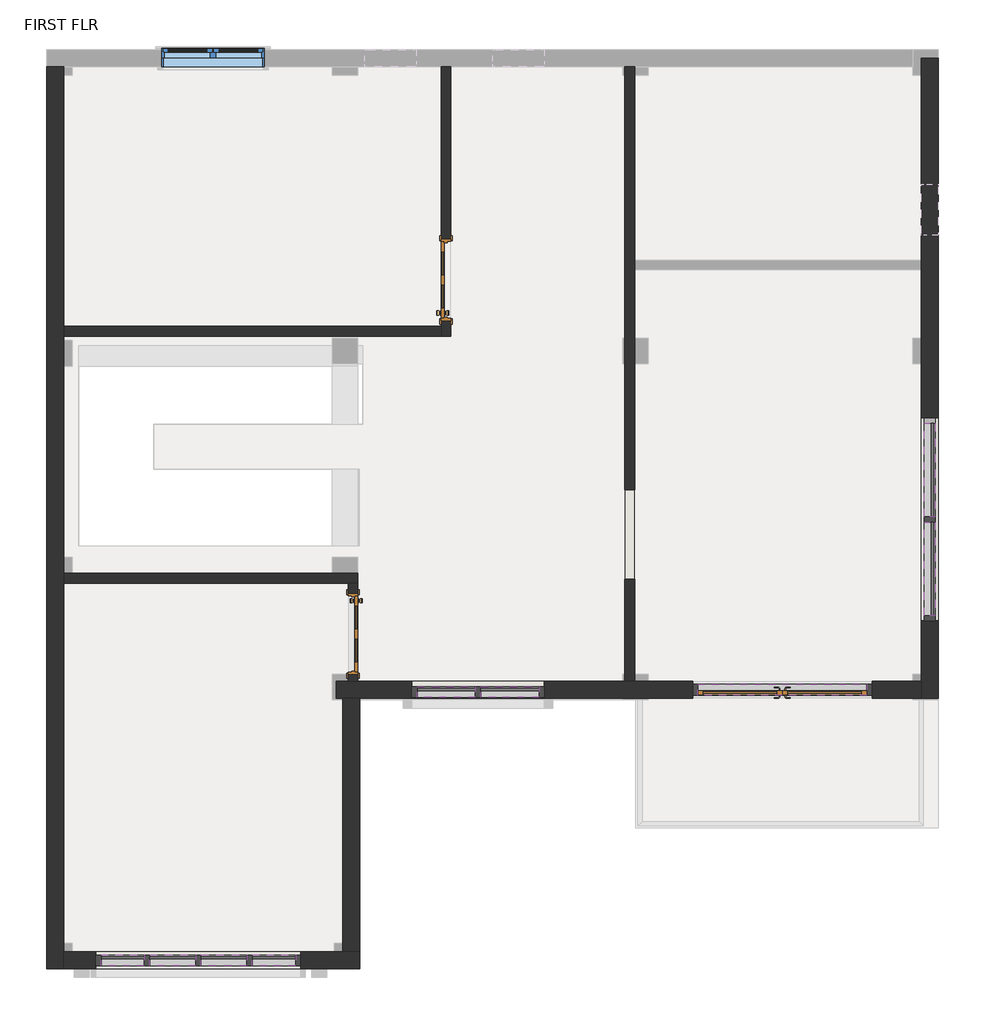
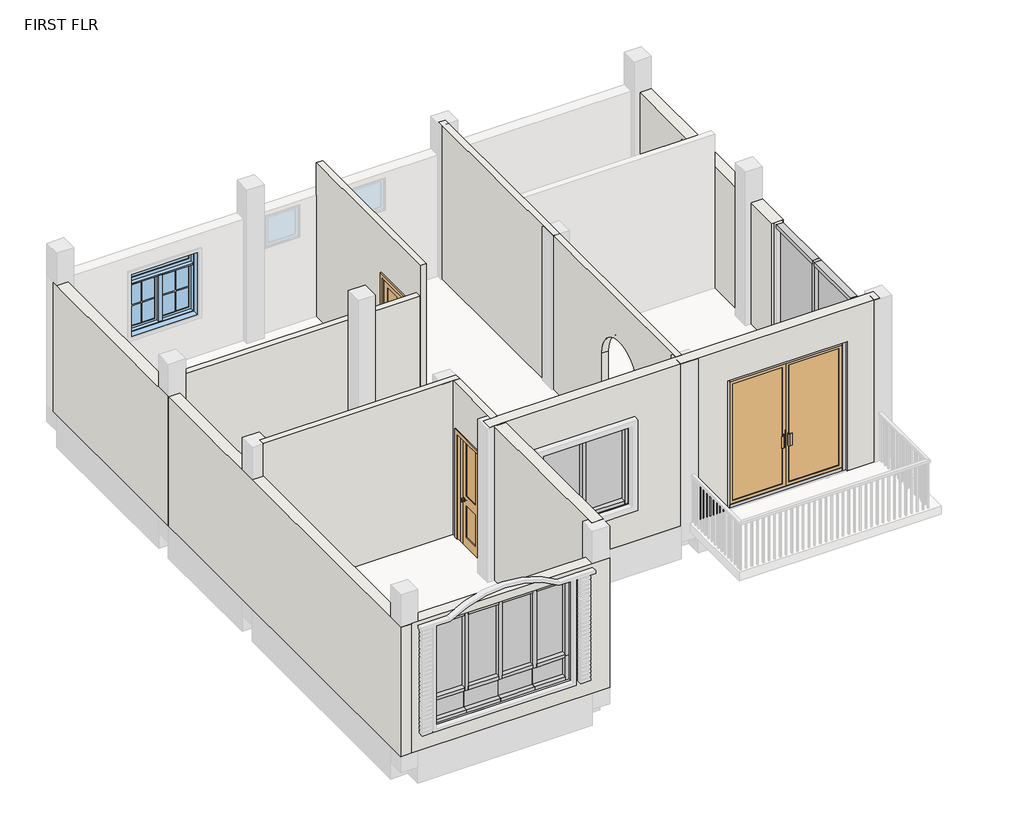
# One storey, part 1 of 3: 37 members, 12 plates, 10 walls, 3 doors, 1 window.
"""IFC4 building model written with IfcOpenShell, lengths in millimetres."""

from ifc_helpers import new_model, si_unit, frame, origin, place, context, project, spatial, polyline, circle_curve, outline, extrude, faceted_brep, transform, mapped, element, save
from ifc_brep_helpers import plane_surface, revolved_surface, advanced_brep
from components import door_curtain_wall_double_storefront_door_curtain_wall_double_726648f4, door_c2926031, member_5f1d7e17, member_aaf6ec4e, member_ee409385, member_16b81337, member_15823cb3, member_aaa03826, member_0b7646a3, member_0a1a1ade, member_a980948f, member_47bfaf8a, member_a27ebcd1, member_a6b28368, member_3586d5c2, member_9c2f0336, member_4d8d05fd, member_5f9244a4, system_panel_glazed_398ce57b, system_panel_glazed_0920ec04, system_panel_glazed_65fa7e48, system_panel_glazed_42028690, system_panel_glazed_d353ffa9, system_panel_glazed_cd98352a, window_ba962a69

model = new_model("IFC4")

# Units and contexts
model_context = context("Model", 3, world=origin())
ifc_project = project(units=[si_unit("LENGTHUNIT", "METRE", prefix="MILLI")], contexts=[model_context])

# Site, building, storey
site = spatial("IfcSite", under=ifc_project)
building = spatial("IfcBuilding", under=site)
storey = spatial("IfcBuildingStorey", under=building, Name="FIRST FLR", Elevation=3352.8)

# Doors
placement = place(None, origin())
door_curtain_wall_double_storefront_door_curtain_wall_double_shape = door_curtain_wall_double_storefront_door_curtain_wall_double_726648f4(model_context)
element("IfcDoor", 1, ObjectType="Door-Curtain-Wall-Double-Storefront : Door-Curtain-Wall-Double-Storefront", at=placement, inside=storey, context=model_context, shape_type="MappedRepresentation", body=[
    mapped(door_curtain_wall_double_storefront_door_curtain_wall_double_shape, transform((-2901.3658472, -10169.7896616, 3416.3), x_axis=(-1.0, 0.0, 0.0), y_axis=(0.0, -1.0, 0.0), z_axis=(0.0, 0.0, 1.0))),
])
door_shape = door_c2926031(model_context)
element("IfcDoor", 2, ObjectType="Door-Interior-Single-4_Panel-Wood : 36\" x 84\"", at=placement, inside=storey, context=model_context, shape_type="MappedRepresentation", body=[
    mapped(door_shape, transform((-6902.1520642, -5299.3396616, 3352.8), x_axis=(0.0, 1.0, 0.0), y_axis=(-1.0, 0.0, 0.0), z_axis=(0.0, 0.0, 1.0))),
])
element("IfcDoor", 3, ObjectType="Door-Interior-Single-4_Panel-Wood : 36\" x 84\"", at=placement, inside=storey, context=model_context, shape_type="MappedRepresentation", body=[
    mapped(door_shape, transform((-8000.7020642, -9507.6885003, 3352.8), x_axis=(0.0, -1.0, 0.0), y_axis=(1.0, 0.0, 0.0), z_axis=(0.0, 0.0, 1.0))),
])

# Members
member_shape = member_5f1d7e17(model_context)
element("IfcMember", 4, ObjectType="Rectangular Mullion : 2.5\" x 5\" rectangular", at=placement, inside=storey, context=model_context, shape_type="MappedRepresentation", body=[
    mapped(member_shape, transform((-5792.9495061, -10198.7950286, 5610.9421259), x_axis=(0.0, 0.0, 1.0), y_axis=(0.0, -1.0, 0.0), z_axis=(1.0, 0.0, 0.0))),
])
element("IfcMember", 5, ObjectType="Rectangular Mullion : 2.5\" x 5\" rectangular", at=placement, inside=storey, context=model_context, shape_type="MappedRepresentation", body=[
    mapped(member_shape, transform((-6548.5995061, -10198.7950286, 5610.9421259), x_axis=(0.0, 0.0, 1.0), y_axis=(0.0, -1.0, 0.0), z_axis=(1.0, 0.0, 0.0))),
])
element("IfcMember", 6, ObjectType="Rectangular Mullion : 2.5\" x 5\" rectangular", at=placement, inside=storey, context=model_context, shape_type="MappedRepresentation", body=[
    mapped(member_shape, transform((-7240.7495061, -10198.7950286, 4104.766106), x_axis=(0.0, 0.0, -1.0), y_axis=(0.0, -1.0, 0.0), z_axis=(-1.0, 0.0, 0.0))),
])
element("IfcMember", 7, ObjectType="Rectangular Mullion : 2.5\" x 5\" rectangular", at=placement, inside=storey, context=model_context, shape_type="MappedRepresentation", body=[
    mapped(member_shape, transform((-6485.0995061, -10198.7950286, 4104.766106), x_axis=(0.0, 0.0, -1.0), y_axis=(0.0, -1.0, 0.0), z_axis=(-1.0, 0.0, 0.0))),
])
member_2_shape = member_aaf6ec4e(model_context)
element("IfcMember", 8, ObjectType="Rectangular Mullion : 2.5\" x 5\" rectangular", at=placement, inside=storey, context=model_context, shape_type="MappedRepresentation", body=[
    mapped(member_2_shape, transform((-1148.7658472, -9288.7247117, 5791.2), x_axis=(0.0, 0.0, 1.0), y_axis=(-1.0, 0.0, 0.0), z_axis=(0.0, -1.0, 0.0))),
])
element("IfcMember", 9, ObjectType="Rectangular Mullion : 2.5\" x 5\" rectangular", at=placement, inside=storey, context=model_context, shape_type="MappedRepresentation", body=[
    mapped(member_2_shape, transform((-1148.7658472, -8113.9747117, 5791.2), x_axis=(0.0, 0.0, 1.0), y_axis=(-1.0, 0.0, 0.0), z_axis=(0.0, -1.0, 0.0))),
])
element("IfcMember", 10, ObjectType="Rectangular Mullion : 2.5\" x 5\" rectangular", at=placement, inside=storey, context=model_context, shape_type="MappedRepresentation", body=[
    mapped(member_2_shape, transform((-1148.7658472, -7002.7247117, 3556.6845972), x_axis=(0.0, 0.0, -1.0), y_axis=(-1.0, 0.0, 0.0), z_axis=(0.0, 1.0, 0.0))),
])
element("IfcMember", 11, ObjectType="Rectangular Mullion : 2.5\" x 5\" rectangular", at=placement, inside=storey, context=model_context, shape_type="MappedRepresentation", body=[
    mapped(member_2_shape, transform((-1148.7658472, -8177.4747117, 3556.6845972), x_axis=(0.0, 0.0, -1.0), y_axis=(-1.0, 0.0, 0.0), z_axis=(0.0, 1.0, 0.0))),
])
member_3_shape = member_ee409385(model_context)
element("IfcMember", 12, ObjectType="Rectangular Mullion : 2.5\" x 5\" rectangular", at=placement, inside=storey, context=model_context, shape_type="MappedRepresentation", body=[
    mapped(member_3_shape, transform((-3968.1658472, -10169.7896616, 3352.8), x_axis=(-1.0, 0.0, 0.0), y_axis=(0.0, 1.0, 0.0), z_axis=(0.0, 0.0, -1.0))),
])
element("IfcMember", 13, ObjectType="Rectangular Mullion : 2.5\" x 5\" rectangular", at=placement, inside=storey, context=model_context, shape_type="MappedRepresentation", body=[
    mapped(member_3_shape, transform((-1834.5658472, -10169.7896616, 5791.2), x_axis=(1.0, 0.0, 0.0), y_axis=(0.0, 1.0, 0.0), z_axis=(0.0, 0.0, 1.0))),
])
member_4_shape = member_16b81337(model_context)
element("IfcMember", 14, ObjectType="Rectangular Mullion : 2.5\" x 5\" rectangular", at=placement, inside=storey, context=model_context, shape_type="MappedRepresentation", body=[
    mapped(member_4_shape, transform((-3904.6658472, -10169.7896616, 5791.2), x_axis=(0.0, 0.0, 1.0), y_axis=(0.0, 1.0, 0.0), z_axis=(-1.0, 0.0, 0.0))),
])
element("IfcMember", 15, ObjectType="Rectangular Mullion : 2.5\" x 5\" rectangular", at=placement, inside=storey, context=model_context, shape_type="MappedRepresentation", body=[
    mapped(member_4_shape, transform((-1898.0658472, -10169.7896616, 3352.8), x_axis=(0.0, 0.0, -1.0), y_axis=(0.0, 1.0, 0.0), z_axis=(1.0, 0.0, 0.0))),
])
member_5_shape = member_15823cb3(model_context)
element("IfcMember", 16, ObjectType="Rectangular Mullion : 2.5\" x 5\" rectangular", at=placement, inside=storey, context=model_context, shape_type="MappedRepresentation", body=[
    mapped(member_5_shape, transform((-8623.1236584, -13386.202305, 3734.1026126), x_axis=(1.0, 0.0, 0.0), y_axis=(0.0, -1.0, 0.0), z_axis=(0.0, 0.0, -1.0))),
])
element("IfcMember", 17, ObjectType="Rectangular Mullion : 2.5\" x 5\" rectangular", at=placement, inside=storey, context=model_context, shape_type="MappedRepresentation", body=[
    mapped(member_5_shape, transform((-11061.5236584, -13386.202305, 4191.3026126), x_axis=(-1.0, 0.0, 0.0), y_axis=(0.0, -1.0, 0.0), z_axis=(0.0, 0.0, 1.0))),
])
member_6_shape = member_aaa03826(model_context)
element("IfcMember", 18, ObjectType="Rectangular Mullion : 2.5\" x 5\" rectangular", at=placement, inside=storey, context=model_context, shape_type="MappedRepresentation", body=[
    mapped(member_6_shape, transform((-10483.6736584, -13386.202305, 4191.3026126), x_axis=(0.0, 0.0, 1.0), y_axis=(0.0, -1.0, 0.0), z_axis=(1.0, 0.0, 0.0))),
])
element("IfcMember", 19, ObjectType="Rectangular Mullion : 2.5\" x 5\" rectangular", at=placement, inside=storey, context=model_context, shape_type="MappedRepresentation", body=[
    mapped(member_6_shape, transform((-8686.6236584, -13386.202305, 4191.3026126), x_axis=(0.0, 0.0, 1.0), y_axis=(0.0, -1.0, 0.0), z_axis=(1.0, 0.0, 0.0))),
])
member_7_shape = member_0b7646a3(model_context)
element("IfcMember", 20, ObjectType="Rectangular Mullion : 2.5\" x 5\" rectangular", at=placement, inside=storey, context=model_context, shape_type="MappedRepresentation", body=[
    mapped(member_7_shape, transform((-8686.6236584, -13386.202305, 5646.3214447), x_axis=(0.0, 0.0, 1.0), y_axis=(0.0, -1.0, 0.0), z_axis=(1.0, 0.0, 0.0))),
])
element("IfcMember", 21, ObjectType="Rectangular Mullion : 2.5\" x 5\" rectangular", at=placement, inside=storey, context=model_context, shape_type="MappedRepresentation", body=[
    mapped(member_7_shape, transform((-10483.6736584, -13386.202305, 5646.3214447), x_axis=(0.0, 0.0, 1.0), y_axis=(0.0, -1.0, 0.0), z_axis=(1.0, 0.0, 0.0))),
])
member_8_shape = member_0a1a1ade(model_context)
element("IfcMember", 22, ObjectType="Rectangular Mullion : 2.5\" x 5\" rectangular", at=placement, inside=storey, context=model_context, shape_type="MappedRepresentation", body=[
    mapped(member_8_shape, transform((-9874.0736584, -13386.202305, 4191.3026126), x_axis=(0.0, 0.0, 1.0), y_axis=(0.0, -1.0, 0.0), z_axis=(1.0, 0.0, 0.0))),
])
element("IfcMember", 23, ObjectType="Rectangular Mullion : 2.5\" x 5\" rectangular", at=placement, inside=storey, context=model_context, shape_type="MappedRepresentation", body=[
    mapped(member_8_shape, transform((-9264.4736584, -13386.202305, 4191.3026126), x_axis=(0.0, 0.0, 1.0), y_axis=(0.0, -1.0, 0.0), z_axis=(1.0, 0.0, 0.0))),
])
element("IfcMember", 24, ObjectType="Rectangular Mullion : 2.5\" x 5\" rectangular", at=placement, inside=storey, context=model_context, shape_type="MappedRepresentation", body=[
    mapped(member_8_shape, transform((-9264.4736584, -13386.202305, 4191.3026126), x_axis=(0.0, 0.0, 1.0), y_axis=(0.0, -1.0, 0.0), z_axis=(1.0, 0.0, 0.0))),
])
member_9_shape = member_a980948f(model_context)
element("IfcMember", 25, ObjectType="Rectangular Mullion : 2.5\" x 5\" rectangular", at=placement, inside=storey, context=model_context, shape_type="MappedRepresentation", body=[
    mapped(member_9_shape, transform((-9874.0736584, -13386.202305, 5646.3214447), x_axis=(0.0, 0.0, 1.0), y_axis=(0.0, -1.0, 0.0), z_axis=(1.0, 0.0, 0.0))),
])
element("IfcMember", 26, ObjectType="Rectangular Mullion : 2.5\" x 5\" rectangular", at=placement, inside=storey, context=model_context, shape_type="MappedRepresentation", body=[
    mapped(member_9_shape, transform((-9264.4736584, -13386.202305, 5646.3214447), x_axis=(0.0, 0.0, 1.0), y_axis=(0.0, -1.0, 0.0), z_axis=(1.0, 0.0, 0.0))),
])
element("IfcMember", 27, ObjectType="Rectangular Mullion : 2.5\" x 5\" rectangular", at=placement, inside=storey, context=model_context, shape_type="MappedRepresentation", body=[
    mapped(member_9_shape, transform((-9232.7236584, -13386.202305, 3734.1026126), x_axis=(0.0, 0.0, -1.0), y_axis=(0.0, -1.0, 0.0), z_axis=(-1.0, 0.0, 0.0))),
])
member_10_shape = member_47bfaf8a(model_context)
element("IfcMember", 28, ObjectType="Rectangular Mullion : 2.5\" x 5\" rectangular", at=placement, inside=storey, context=model_context, shape_type="MappedRepresentation", body=[
    mapped(member_10_shape, transform((-10451.9236584, -13386.202305, 3734.1026126), x_axis=(0.0, 0.0, -1.0), y_axis=(0.0, -1.0, 0.0), z_axis=(-1.0, 0.0, 0.0))),
])
element("IfcMember", 29, ObjectType="Rectangular Mullion : 2.5\" x 5\" rectangular", at=placement, inside=storey, context=model_context, shape_type="MappedRepresentation", body=[
    mapped(member_10_shape, transform((-9842.3236584, -13386.202305, 3734.1026126), x_axis=(0.0, 0.0, -1.0), y_axis=(0.0, -1.0, 0.0), z_axis=(-1.0, 0.0, 0.0))),
])
element("IfcMember", 30, ObjectType="Rectangular Mullion : 2.5\" x 5\" rectangular", at=placement, inside=storey, context=model_context, shape_type="MappedRepresentation", body=[
    mapped(member_9_shape, transform((-10998.0236584, -13386.202305, 3734.1026126), x_axis=(0.0, 0.0, -1.0), y_axis=(0.0, -1.0, 0.0), z_axis=(-1.0, 0.0, 0.0))),
])
member_11_shape = member_a27ebcd1(model_context)
element("IfcMember", 31, ObjectType="Rectangular Mullion : 2.5\" x 5\" rectangular", at=placement, inside=storey, context=model_context, shape_type="MappedRepresentation", body=[
    mapped(member_11_shape, transform((-10451.9236584, -13386.202305, 4159.5526126), x_axis=(1.0, 0.0, 0.0), y_axis=(0.0, -1.0, 0.0), z_axis=(0.0, 0.0, -1.0))),
])
element("IfcMember", 32, ObjectType="Rectangular Mullion : 2.5\" x 5\" rectangular", at=placement, inside=storey, context=model_context, shape_type="MappedRepresentation", body=[
    mapped(member_11_shape, transform((-9842.3236584, -13386.202305, 4159.5526126), x_axis=(1.0, 0.0, 0.0), y_axis=(0.0, -1.0, 0.0), z_axis=(0.0, 0.0, -1.0))),
])
element("IfcMember", 33, ObjectType="Rectangular Mullion : 2.5\" x 5\" rectangular", at=placement, inside=storey, context=model_context, shape_type="MappedRepresentation", body=[
    mapped(member_11_shape, transform((-9232.7236584, -13386.202305, 4159.5526126), x_axis=(1.0, 0.0, 0.0), y_axis=(0.0, -1.0, 0.0), z_axis=(0.0, 0.0, -1.0))),
])
member_12_shape = member_a6b28368(model_context)
element("IfcMember", 34, ObjectType="Rectangular Mullion : 2.5\" x 5\" rectangular", at=placement, inside=storey, context=model_context, shape_type="MappedRepresentation", body=[
    mapped(member_12_shape, transform((-11061.5236584, -13386.202305, 5646.3214447), x_axis=(-1.0, 0.0, 0.0), y_axis=(0.0, -1.0, 0.0), z_axis=(0.0, 0.0, 1.0))),
])
element("IfcMember", 35, ObjectType="Rectangular Mullion : 2.5\" x 5\" rectangular", at=placement, inside=storey, context=model_context, shape_type="MappedRepresentation", body=[
    mapped(member_12_shape, transform((-8623.1236584, -13386.202305, 4191.3026126), x_axis=(1.0, 0.0, 0.0), y_axis=(0.0, -1.0, 0.0), z_axis=(0.0, 0.0, -1.0))),
])
member_13_shape = member_3586d5c2(model_context)
element("IfcMember", 36, ObjectType="Rectangular Mullion : 2.5\" x 5\" rectangular", at=placement, inside=storey, context=model_context, shape_type="MappedRepresentation", body=[
    mapped(member_13_shape, transform((-6516.8495061, -10198.7950286, 4104.766106), x_axis=(1.0, 0.0, 0.0), y_axis=(0.0, -1.0, 0.0), z_axis=(0.0, 0.0, -1.0))),
])
member_14_shape = member_9c2f0336(model_context)
element("IfcMember", 37, ObjectType="Rectangular Mullion : 2.5\" x 5\" rectangular", at=placement, inside=storey, context=model_context, shape_type="MappedRepresentation", body=[
    mapped(member_14_shape, transform((-5729.4495061, -10198.7950286, 4104.766106), x_axis=(1.0, 0.0, 0.0), y_axis=(0.0, -1.0, 0.0), z_axis=(0.0, 0.0, -1.0))),
])
element("IfcMember", 38, ObjectType="Rectangular Mullion : 2.5\" x 5\" rectangular", at=placement, inside=storey, context=model_context, shape_type="MappedRepresentation", body=[
    mapped(member_14_shape, transform((-7304.2495061, -10198.7950286, 5610.9421259), x_axis=(-1.0, 0.0, 0.0), y_axis=(0.0, -1.0, 0.0), z_axis=(0.0, 0.0, 1.0))),
])
member_15_shape = member_4d8d05fd(model_context)
element("IfcMember", 39, ObjectType="Rectangular Mullion : 2.5\" x 5\" rectangular", at=placement, inside=storey, context=model_context, shape_type="MappedRepresentation", body=[
    mapped(member_15_shape, transform((-1148.7658472, -8145.7247117, 3556.6845972), x_axis=(0.0, -1.0, 0.0), y_axis=(-1.0, 0.0, 0.0), z_axis=(0.0, 0.0, -1.0))),
])
member_16_shape = member_5f9244a4(model_context)
element("IfcMember", 40, ObjectType="Rectangular Mullion : 2.5\" x 5\" rectangular", at=placement, inside=storey, context=model_context, shape_type="MappedRepresentation", body=[
    mapped(member_16_shape, transform((-1148.7658472, -9352.2247117, 3556.6845972), x_axis=(0.0, -1.0, 0.0), y_axis=(-1.0, 0.0, 0.0), z_axis=(0.0, 0.0, -1.0))),
])

# Plates
system_panel_glazed_shape = system_panel_glazed_398ce57b(model_context)
element("IfcPlate", 41, ObjectType="System Panel : Glazed", at=placement, inside=storey, context=model_context, shape_type="MappedRepresentation", body=[
    mapped(system_panel_glazed_shape, transform((-10724.9736584, -13386.202305, 3797.6026126), x_axis=(1.0, 0.0, 0.0), y_axis=(0.0, 1.0, 0.0), z_axis=(0.0, 0.0, 1.0))),
])
element("IfcPlate", 42, ObjectType="System Panel : Glazed", at=placement, inside=storey, context=model_context, shape_type="MappedRepresentation", body=[
    mapped(system_panel_glazed_shape, transform((-8959.6736584, -13386.202305, 3797.6026126), x_axis=(1.0, 0.0, 0.0), y_axis=(0.0, 1.0, 0.0), z_axis=(0.0, 0.0, 1.0))),
])
system_panel_glazed_2_shape = system_panel_glazed_0920ec04(model_context)
element("IfcPlate", 43, ObjectType="System Panel : Glazed", at=placement, inside=storey, context=model_context, shape_type="MappedRepresentation", body=[
    mapped(system_panel_glazed_2_shape, transform((-10147.1236584, -13386.202305, 3797.6026126), x_axis=(1.0, 0.0, 0.0), y_axis=(0.0, 1.0, 0.0), z_axis=(0.0, 0.0, 1.0))),
])
element("IfcPlate", 44, ObjectType="System Panel : Glazed", at=placement, inside=storey, context=model_context, shape_type="MappedRepresentation", body=[
    mapped(system_panel_glazed_2_shape, transform((-9537.5236584, -13386.202305, 3797.6026126), x_axis=(1.0, 0.0, 0.0), y_axis=(0.0, 1.0, 0.0), z_axis=(0.0, 0.0, 1.0))),
])
system_panel_glazed_3_shape = system_panel_glazed_65fa7e48(model_context)
element("IfcPlate", 45, ObjectType="System Panel : Glazed", at=placement, inside=storey, context=model_context, shape_type="MappedRepresentation", body=[
    mapped(system_panel_glazed_3_shape, transform((-10740.8486584, -13386.202305, 4223.0526126), x_axis=(1.0, 0.0, 0.0), y_axis=(0.0, 1.0, 0.0), z_axis=(0.0, 0.0, 1.0))),
])
element("IfcPlate", 46, ObjectType="System Panel : Glazed", at=placement, inside=storey, context=model_context, shape_type="MappedRepresentation", body=[
    mapped(system_panel_glazed_3_shape, transform((-8943.7986584, -13386.202305, 4223.0526126), x_axis=(1.0, 0.0, 0.0), y_axis=(0.0, 1.0, 0.0), z_axis=(0.0, 0.0, 1.0))),
])
system_panel_glazed_4_shape = system_panel_glazed_42028690(model_context)
element("IfcPlate", 47, ObjectType="System Panel : Glazed", at=placement, inside=storey, context=model_context, shape_type="MappedRepresentation", body=[
    mapped(system_panel_glazed_4_shape, transform((-10147.1236584, -13386.202305, 4223.0526126), x_axis=(1.0, 0.0, 0.0), y_axis=(0.0, 1.0, 0.0), z_axis=(0.0, 0.0, 1.0))),
])
element("IfcPlate", 48, ObjectType="System Panel : Glazed", at=placement, inside=storey, context=model_context, shape_type="MappedRepresentation", body=[
    mapped(system_panel_glazed_4_shape, transform((-9537.5236584, -13386.202305, 4223.0526126), x_axis=(1.0, 0.0, 0.0), y_axis=(0.0, 1.0, 0.0), z_axis=(0.0, 0.0, 1.0))),
])
system_panel_glazed_5_shape = system_panel_glazed_d353ffa9(model_context)
element("IfcPlate", 49, ObjectType="System Panel : Glazed", at=placement, inside=storey, context=model_context, shape_type="MappedRepresentation", body=[
    mapped(system_panel_glazed_5_shape, transform((-6894.6745061, -10198.7950286, 4168.266106), x_axis=(1.0, 0.0, 0.0), y_axis=(0.0, 1.0, 0.0), z_axis=(0.0, 0.0, 1.0))),
])
element("IfcPlate", 50, ObjectType="System Panel : Glazed", at=placement, inside=storey, context=model_context, shape_type="MappedRepresentation", body=[
    mapped(system_panel_glazed_5_shape, transform((-6139.0245061, -10198.7950286, 4168.266106), x_axis=(1.0, 0.0, 0.0), y_axis=(0.0, 1.0, 0.0), z_axis=(0.0, 0.0, 1.0))),
])
system_panel_glazed_6_shape = system_panel_glazed_cd98352a(model_context)
element("IfcPlate", 51, ObjectType="System Panel : Glazed", at=placement, inside=storey, context=model_context, shape_type="MappedRepresentation", body=[
    mapped(system_panel_glazed_6_shape, transform((-1148.7658472, -7558.3497117, 3620.1845972), x_axis=(0.0, -1.0, 0.0), y_axis=(1.0, 0.0, 0.0), z_axis=(0.0, 0.0, 1.0))),
])
element("IfcPlate", 52, ObjectType="System Panel : Glazed", at=placement, inside=storey, context=model_context, shape_type="MappedRepresentation", body=[
    mapped(system_panel_glazed_6_shape, transform((-1148.7658472, -8733.0997117, 3620.1845972), x_axis=(0.0, -1.0, 0.0), y_axis=(1.0, 0.0, 0.0), z_axis=(0.0, 0.0, 1.0))),
])

# Walls
element("IfcWall", 53, ObjectType="EXTERIOR 8'", at=placement, inside=storey, context=model_context, shape_type="Brep", body=[
    faceted_brep([(-1250.3658472, -2665.6747117, 3352.8), (-1250.3658472, -5064.3896616, 3352.8), (-1250.3658472, -5178.6896616, 3352.8), (-1250.3658472, -10068.1896616, 3352.8), (-1250.3658472, -10271.3896616, 3352.8), (-1250.3658472, -10271.3896616, 5791.2), (-1250.3658472, -9352.2247117, 5791.2), (-1250.3658472, -9352.2247117, 3556.6845972), (-1250.3658472, -6939.2247117, 3556.6845972), (-1250.3658472, -6939.2247117, 5791.2), (-1250.3658472, -2665.6747117, 5791.2), (-1250.3658472, -4769.9071866, 5689.6), (-1250.3658472, -4769.9071866, 5080.0), (-1250.3658472, -4160.3071866, 5080.0), (-1250.3658472, -4160.3071866, 5689.6), (-1047.1658472, -10271.3896616, 3352.8), (-1047.1658472, -2665.6747117, 3352.8), (-1047.1658472, -2665.6747117, 5791.2), (-1047.1658472, -6939.2247117, 5791.2), (-1047.1658472, -6939.2247117, 3556.6845972), (-1047.1658472, -9352.2247117, 3556.6845972), (-1047.1658472, -9352.2247117, 5791.2), (-1047.1658472, -10271.3896616, 5791.2), (-1047.1658472, -4769.9071866, 5080.0), (-1047.1658472, -4769.9071866, 5689.6), (-1047.1658472, -4160.3071866, 5689.6), (-1047.1658472, -4160.3071866, 5080.0)], [[[0, 1, 2, 3, 4, 5, 6, 7, 8, 9, 10], [11, 12, 13, 14]], [[15, 16, 17, 18, 19, 20, 21, 22], [23, 24, 25, 26]], [[4, 3, 2, 1, 0, 16, 15]], [[17, 10, 9, 18]], [[5, 22, 21, 6]], [[0, 10, 17, 16]], [[5, 4, 15, 22]], [[8, 19, 18, 9]], [[20, 7, 6, 21]], [[19, 8, 7, 20]], [[11, 24, 23, 12]], [[12, 23, 26, 13]], [[13, 26, 25, 14]], [[24, 11, 14, 25]]]),
])
element("IfcWall", 54, ObjectType="EXTERIOR 8'", at=placement, inside=storey, context=model_context, shape_type="Brep", body=[
    faceted_brep([(-11645.7236584, -2767.2747117, 3352.8), (-11645.7236584, -13487.802305, 3352.8), (-11645.7236584, -13487.802305, 5787.4119669), (-11645.7236584, -2767.2747117, 5787.4119669), (-11442.5236584, -2767.2747117, 3352.8), (-11442.5236584, -2767.2747117, 5787.4119669), (-11442.5236584, -13487.802305, 5787.4119669), (-11442.5236584, -13487.802305, 3352.8), (-11442.5236584, -13284.602305, 3352.8), (-11442.5236584, -8902.7373391, 3352.8), (-11442.5236584, -8788.4373391, 3352.8), (-11442.5236584, -5966.0896616, 3352.8), (-11442.5236584, -5851.7896616, 3352.8)], [[[0, 1, 2, 3]], [[4, 5, 6, 7, 8, 9, 10, 11, 12]], [[1, 0, 4, 12, 11, 10, 9, 8, 7]], [[3, 2, 6, 5]], [[0, 3, 5, 4]], [[2, 1, 7, 6]]]),
])
element("IfcWall", 55, ObjectType="EXTERIOR 8'", at=placement, inside=storey, context=model_context, shape_type="Brep", body=[
    faceted_brep([(-1250.3658472, -10271.3896616, 6400.8), (-7921.3270642, -10271.3896616, 6400.8), (-8124.5270642, -10271.3896616, 6400.8), (-8200.7270642, -10271.3896616, 6400.8), (-8200.7270642, -10271.3896616, 3352.8), (-8124.5270642, -10271.3896616, 3352.8), (-7921.3270642, -10271.3896616, 3352.8), (-3968.1658472, -10271.3896616, 3352.8), (-3968.1658472, -10271.3896616, 5791.2), (-1834.5658472, -10271.3896616, 5791.2), (-1834.5658472, -10271.3896616, 3352.8), (-1250.3658472, -10271.3896616, 3352.8), (-1250.3658472, -10271.3896616, 5791.2), (-7304.2495061, -10271.3896616, 4104.766106), (-7304.2495061, -10271.3896616, 5610.9421259), (-5729.4495061, -10271.3896616, 5610.9421259), (-5729.4495061, -10271.3896616, 4104.766106), (-8200.7270642, -10068.1896616, 6400.8), (-8061.0270642, -10068.1896616, 6400.8), (-7946.7270642, -10068.1896616, 6400.8), (-4771.7270642, -10068.1896616, 6400.8), (-4657.4270642, -10068.1896616, 6400.8), (-1250.3658472, -10068.1896616, 6400.8), (-1250.3658472, -10068.1896616, 3352.8), (-1834.5658472, -10068.1896616, 3352.8), (-1834.5658472, -10068.1896616, 5791.2), (-3968.1658472, -10068.1896616, 5791.2), (-3968.1658472, -10068.1896616, 3352.8), (-4657.4270642, -10068.1896616, 3352.8), (-4771.7270642, -10068.1896616, 3352.8), (-7946.7270642, -10068.1896616, 3352.8), (-8061.0270642, -10068.1896616, 3352.8), (-8200.7270642, -10068.1896616, 3352.8), (-7304.2495061, -10068.1896616, 5610.9421259), (-7304.2495061, -10068.1896616, 4104.766106), (-5729.4495061, -10068.1896616, 4104.766106), (-5729.4495061, -10068.1896616, 5610.9421259)], [[[0, 1, 2, 3, 4, 5, 6, 7, 8, 9, 10, 11, 12], [13, 14, 15, 16]], [[17, 18, 19, 20, 21, 22, 23, 24, 25, 26, 27, 28, 29, 30, 31, 32], [33, 34, 35, 36]], [[4, 32, 31, 30, 29, 28, 27, 7, 6, 5]], [[23, 11, 10, 24]], [[3, 2, 1, 0, 22, 21, 20, 19, 18, 17]], [[4, 3, 17, 32]], [[0, 12, 11, 23, 22]], [[13, 34, 33, 14]], [[14, 33, 36, 15]], [[15, 36, 35, 16]], [[34, 13, 16, 35]], [[9, 25, 24, 10]], [[25, 9, 8, 26]], [[26, 8, 7, 27]]]),
])
element("IfcWall", 56, ObjectType="EXTERIOR 8'", at=placement, inside=storey, context=model_context, shape_type="Brep", body=[
    faceted_brep([(-11442.5236584, -13487.802305, 3352.8), (-7921.3270642, -13487.802305, 3352.8), (-7921.3270642, -13487.802305, 5791.2), (-11442.5236584, -13487.802305, 5791.2), (-11442.5236584, -13487.802305, 5787.4119669), (-11061.5236584, -13487.802305, 3734.1026126), (-11061.5236584, -13487.802305, 5646.3214447), (-8623.1236584, -13487.802305, 5646.3214447), (-8623.1236584, -13487.802305, 3734.1026126), (-7921.3270642, -13284.602305, 3352.8), (-8124.5270642, -13284.602305, 3352.8), (-11442.5236584, -13284.602305, 3352.8), (-11442.5236584, -13284.602305, 5791.2), (-7921.3270642, -13284.602305, 5791.2), (-11061.5236584, -13284.602305, 5646.3214447), (-11061.5236584, -13284.602305, 3734.1026126), (-8623.1236584, -13284.602305, 3734.1026126), (-8623.1236584, -13284.602305, 5646.3214447)], [[[0, 1, 2, 3, 4], [5, 6, 7, 8]], [[9, 10, 11, 12, 13], [14, 15, 16, 17]], [[1, 0, 11, 10, 9]], [[3, 2, 13, 12]], [[0, 4, 3, 12, 11]], [[2, 1, 9, 13]], [[5, 15, 14, 6]], [[6, 14, 17, 7]], [[7, 17, 16, 8]], [[15, 5, 8, 16]]]),
])
element("IfcWall", 57, ObjectType="EXTERIOR 8'", at=placement, inside=storey, context=model_context, shape_type="Brep", body=[
    faceted_brep([(-7921.3270642, -13284.602305, 3352.8), (-7921.3270642, -10271.3896616, 3352.8), (-7921.3270642, -10271.3896616, 6400.8), (-7921.3270642, -13284.602305, 6400.8), (-7921.3270642, -13284.602305, 5791.2), (-8124.5270642, -13284.602305, 3352.8), (-8124.5270642, -13284.602305, 6400.8), (-8124.5270642, -10271.3896616, 6400.8), (-8124.5270642, -10271.3896616, 3352.8)], [[[0, 1, 2, 3, 4]], [[5, 6, 7, 8]], [[1, 0, 5, 8]], [[3, 2, 7, 6]], [[0, 4, 3, 6, 5]], [[2, 1, 8, 7]]]),
])
element("IfcWall", 58, ObjectType="interior wall 4.5\"", at=placement, inside=storey, context=model_context, shape_type="Brep", body=[
    faceted_brep([(-6956.1270642, -5966.0896616, 6400.8), (-6956.1270642, -2767.2747117, 6400.8), (-6956.1270642, -2767.2747117, 3352.8), (-6956.1270642, -4816.7396616, 3352.8), (-6956.1270642, -4816.7396616, 5511.8), (-6956.1270642, -5781.9396616, 5511.8), (-6956.1270642, -5781.9396616, 3352.8), (-6956.1270642, -5851.7896616, 3352.8), (-6956.1270642, -5966.0896616, 3352.8), (-6956.1270642, -5966.0896616, 5824.7676537), (-6841.8270642, -2767.2747117, 6400.8), (-6841.8270642, -5966.0896616, 6400.8), (-6841.8270642, -5966.0896616, 3352.8), (-6841.8270642, -5781.9396616, 3352.8), (-6841.8270642, -5781.9396616, 5511.8), (-6841.8270642, -4816.7396616, 5511.8), (-6841.8270642, -4816.7396616, 3352.8), (-6841.8270642, -2767.2747117, 3352.8)], [[[0, 1, 2, 3, 4, 5, 6, 7, 8, 9]], [[10, 11, 12, 13, 14, 15, 16, 17]], [[2, 17, 16, 3]], [[12, 8, 7, 6, 13]], [[1, 0, 11, 10]], [[2, 1, 10, 17]], [[0, 9, 8, 12, 11]], [[15, 4, 3, 16]], [[4, 15, 14, 5]], [[5, 14, 13, 6]]]),
])
element("IfcWall", 59, ObjectType="interior wall 4.5\"", at=placement, inside=storey, context=model_context, shape_type="SweptSolid", body=[
    extrude(outline(polyline([(-11442.5236584, -5851.7896616), (-6956.1270642, -5851.7896616), (-6956.1270642, -5966.0896616), (-11442.5236584, -5966.0896616), (-11442.5236584, -5851.7896616)])), frame((0.0, 0.0, 3352.8), z_axis=(0.0, 0.0, 1.0), x_axis=(1.0, 0.0, 0.0)), (0.0, 0.0, 1.0), 2471.9676537),
])
element("IfcWall", 60, ObjectType="interior wall 4.5\"", at=placement, inside=storey, context=model_context, shape_type="AdvancedBrep", body=[
    advanced_brep(
    [(-4771.7270642, -2767.2747117, 3352.8), (-4771.7270642, -10068.1896616, 3352.8), (-4771.7270642, -10068.1896616, 6400.8), (-4771.7270642, -2767.2747117, 6400.8), (-4771.7270642, -7792.9016001, 5095.1482601), (-4771.7270642, -8859.7016001, 5095.1482601), (-4771.7270642, -8859.7016001, 3367.9482601), (-4771.7270642, -7792.9016001, 3367.9482601), (-4657.4270642, -2767.2747117, 3352.8), (-4657.4270642, -2767.2747117, 6400.8), (-4657.4270642, -5064.3896616, 6400.8), (-4657.4270642, -5178.6896616, 6400.8), (-4657.4270642, -10068.1896616, 6400.8), (-4657.4270642, -10068.1896616, 3352.8), (-4657.4270642, -5178.6896616, 3352.8), (-4657.4270642, -5064.3896616, 3352.8), (-4657.4270642, -7792.9016001, 5095.1482601), (-4657.4270642, -7792.9016001, 3367.9482601), (-4657.4270642, -8859.7016001, 3367.9482601), (-4657.4270642, -8859.7016001, 5095.1482601)],
    [
        (0, 1),
        (1, 2),
        (2, 3),
        (3, 0),
        (4, 5, circle_curve(frame((-4771.7270642, -8326.3016001, 5095.1482601), z_axis=(1.0, 0.0, 0.0), x_axis=(0.0, 1.0, 0.0)), 533.4)),
        (5, 6),
        (6, 7),
        (7, 4),
        (8, 9),
        (9, 10),
        (10, 11),
        (11, 12),
        (12, 13),
        (13, 14),
        (14, 15),
        (15, 8),
        (16, 17),
        (17, 18),
        (18, 19),
        (19, 16, circle_curve(frame((-4657.4270642, -8326.3016001, 5095.1482601), z_axis=(-1.0, 0.0, 0.0), x_axis=(0.0, 1.0, 0.0)), 533.4)),
        (3, 9),
        (8, 0),
        (1, 13),
        (12, 2),
        (4, 16),
        (19, 5),
        (18, 6),
        (17, 7),
    ],
    [
        plane_surface(frame((-4771.7270642, -2803.7896616, 3352.8), z_axis=(-1.0, 0.0, 0.0), x_axis=(0.0, -1.0, 0.0))),
        plane_surface(frame((-4657.4270642, -2803.7896616, 3352.8), z_axis=(1.0, 0.0, 0.0), x_axis=(0.0, 1.0, 0.0))),
        plane_surface(frame((-11624.0070023, -2767.2747117, 3352.8), z_axis=(0.0, 1.0, 0.0), x_axis=(1.0, 0.0, 0.0))),
        plane_surface(frame((-8013.5236584, -10068.1896616, 3352.8), z_axis=(0.0, -1.0, 0.0), x_axis=(-1.0, 0.0, 0.0))),
        plane_surface(frame((-4771.7270642, -2665.6747117, 3352.8), z_axis=(0.0, 0.0, -1.0), x_axis=(1.0, 0.0, 0.0))),
        plane_surface(frame((-4771.7270642, -10169.7896616, 6400.8), z_axis=(0.0, 0.0, 1.0), x_axis=(1.0, 0.0, 0.0))),
        revolved_surface(polyline([(-4657.4270642, -7792.9016001, 5095.1482601), (-4771.7270642, -7792.9016001, 5095.1482601)]), (-4714.5770642, -8326.3016001, 5095.1482601), (1.0, 0.0, 0.0)),
        plane_surface(frame((-4771.7270642, -8859.7016001, 5095.1482601), z_axis=(0.0, 1.0, 0.0), x_axis=(1.0, 0.0, 0.0))),
        plane_surface(frame((-4771.7270642, -8859.7016001, 3367.9482601), z_axis=(0.0, 0.0, 1.0), x_axis=(1.0, 0.0, 0.0))),
        plane_surface(frame((-4771.7270642, -7792.9016001, 3367.9482601), z_axis=(0.0, -1.0, 0.0), x_axis=(1.0, 0.0, 0.0))),
    ],
    [
        (0, [[1, 2, 3, 4], [5, 6, 7, 8]]),
        (1, [[9, 10, 11, 12, 13, 14, 15, 16], [17, 18, 19, 20]]),
        (2, [[-4, 21, -9, 22]]),
        (3, [[-2, 23, -13, 24]]),
        (4, [[-1, -22, -16, -15, -14, -23]]),
        (5, [[-3, -24, -12, -11, -10, -21]]),
        (6, [[-5, 25, -20, 26]]),
        (7, [[-6, -26, -19, 27]]),
        (8, [[-7, -27, -18, 28]]),
        (9, [[-8, -28, -17, -25]]),
    ],
),
])
element("IfcWall", 61, ObjectType="interior wall 4.5\"", at=placement, inside=storey, context=model_context, shape_type="Brep", body=[
    faceted_brep([(-11442.5236584, -8902.7373391, 3352.8), (-8061.0270642, -8902.7373391, 3352.8), (-7946.7270642, -8902.7373391, 3352.8), (-7946.7270642, -8902.7373391, 6400.8), (-8061.0270642, -8902.7373391, 6400.8), (-11442.5236584, -8902.7373391, 6400.8), (-11442.5236584, -8788.4373391, 3352.8), (-11442.5236584, -8788.4373391, 6400.8), (-7946.7270642, -8788.4373391, 6400.8), (-7946.7270642, -8788.4373391, 3352.8)], [[[0, 1, 2, 3, 4, 5]], [[6, 7, 8, 9]], [[2, 1, 0, 6, 9]], [[5, 4, 3, 8, 7]], [[0, 5, 7, 6]], [[3, 2, 9, 8]]]),
])
element("IfcWall", 62, ObjectType="interior wall 4.5\"", at=placement, inside=storey, context=model_context, shape_type="SweptSolid", body=[
    extrude(outline(polyline([(-10068.1896616, 6400.8), (-8902.7373391, 6400.8), (-8902.7373391, 3352.8), (-9025.0885003, 3352.8), (-9025.0885003, 5511.8), (-9990.2885003, 5511.8), (-9990.2885003, 3352.8), (-10068.1896616, 3352.8), (-10068.1896616, 6400.8)])), frame((-8061.0270642, 0.0, 0.0), z_axis=(1.0, 0.0, 0.0), x_axis=(0.0, 1.0, 0.0)), (0.0, 0.0, 1.0), 114.3),
])

# Window
window_shape = window_ba962a69(model_context)
element("IfcWindow", 63, ObjectType="Window-Casement-Double-Transom : 48\" x 48\"", at=placement, inside=storey, context=model_context, shape_type="MappedRepresentation", body=[
    mapped(window_shape, transform((-9667.5770642, -2665.6747117, 3352.8), x_axis=(1.0, 0.0, 0.0), y_axis=(0.0, 1.0, 0.0), z_axis=(0.0, 0.0, 1.0))),
])

save(model, "model.ifc")

# Revit data of these elements
# Type "Door-Curtain-Wall-Double-Storefront : Door-Curtain-Wall-Double-Storefront"
#   Type Mark = "9"
#   Construction Type Id = "opn-d46"
#   Assembly Code = "B2030100"
#   Analytic Construction = "Metal frame, double glass door"
#   Width [instance default] = 6' - 0"
#   Thermal Resistance (R) = 1.3794 (h·ft²·°F)/BTU
#   Swing Angle [instance default] = 90.00°
#   Panel Width [instance default] = 3' - 0"
#   Offset = 0' - 2 1/4"
#   Heat Transfer Coefficient (U) = 0.7250 BTU/(h·ft²·°F)
#   Define Thermal Properties by = 1
#   Function = 1
#   Frame Material = Aluminum
#   Door Handle Material = Aluminum
#   Glazing = Glass
#   Visual Light Transmittance = 0
#   Solar Heat Gain Coefficient = 0
# Type "Door-Interior-Single-4_Panel-Wood : 36\" x 84\""
#   Type Mark = "8"
#   Assembly Code = "C1020300"
#   Analytic Construction = "Wooden"
#   Top Rail = 0' - 4 11/16"
#   Thickness = 0' - 1 3/8"
#   Thermal Resistance (R) = 2.5876 (h·ft²·°F)/BTU
#   Swing Angle [instance default] = 90.00°
#   Stiles = 0' - 4 3/4"
#   Rough Width = 3' - 2"
#   Rough Height = 7' - 1"
#   Mullion = 0' - 4 1/2"
#   Lock Rail = 0' - 7 1/2"
#   Height = 7' - 0"
#   Width = 3' - 0"
#   Heat Transfer Coefficient (U) = 0.3865 BTU/(h·ft²·°F)
#   Bottom Rail = 0' - 9 1/8"
#   Trim Material = Cherry
#   Panel Material = Cherry
#   Frame Material = Cherry
#   Door Handle Material = Aluminum
#   Visual Light Transmittance = 0
#   Solar Heat Gain Coefficient = 0
#   Wall Closure = (empty or 0)
#   Function = (empty or 0)
# Type "Rectangular Mullion : 2.5\" x 5\" rectangular"
#   built-in parameter 1007304 = 0.416667 (stored number, unit not read)
#   built-in parameter 1007301 = 0.104167 (stored number, unit not read)
#   built-in parameter 1007300 = 0.104167 (stored number, unit not read)
# Type "System Panel : Glazed"
#   Construction Type Id = "GSP4R"
#   Analytic Construction = "1/8 in Pilkington single glazing"
#   Visual Light Transmittance = 0.9
#   Solar Heat Gain Coefficient = 0.86
#   Heat Transfer Coefficient (U) = 1.18115 BTU/(h·ft²·°F)
#   Define Thermal Properties by = 1
# Type "EXTERIOR 8'"
#   Assembly Code = "B2010"
#   Layers, outside or top first: 0' - 8" "beige colour" (function 1)
# Type "interior wall 4.5\""
#   Assembly Code = "B2010"
#   Layers, outside or top first: 0' - 4 1/2" "beige colour" (function 1)
# Type "Window-Casement-Double-Transom : 48\" x 48\""
#   Type Mark = "18"
#   Fire Rating = "0.5h"
#   Assembly Code = "B2020100"
#   Analytic Construction = "Double glazing - domestic"
#   Window Inset [instance default] = 0' - 0"
#   Wall Thickness [instance default] = 0' - 6"
#   Interior Wall Closure [instance default] = 0' - 2 1/4"
#   Half Width = 2' - 0"
#   Visual Light Transmittance = 0.81
#   Transom Height = 1' - 0"
#   Thermal Resistance (R) = 1.8146 (h·ft²·°F)/BTU
#   Solar Heat Gain Coefficient = 0.76
#   Rough Width = 4' - 0 1/2"
#   Rough Height = 4' - 0 1/2"
#   Open Window Height = 3' - 0"
#   Height = 4' - 0"
#   Heat Transfer Coefficient (U) = 0.5511 BTU/(h·ft²·°F)
#   Frame Extension [instance default] = 0' - 0 1/4"
#   Exterior Wall Closure [instance default] = 0' - 1 1/4"
#   Extension Jamb [instance default] = 0' - 2 1/4"
#   Default Sill Height = 3' - 0"
#   Width = 4' - 0"
#   Muntin Visibility = yes
#   Interior Trim Visibility [instance default] = yes
#   Exterior Trim Visibility [instance default] = yes
#   Extension Jamb Visibility [instance default] = yes
#   Interior Trim Material = Wood - Stained
#   Muntin Pattern = Muntin Pattern_2x2 : Muntin Pattern_2x2
#   Interior Trim = Trim-Window-Interior-Flat : Picture Frame
#   Interior Frame Material = Wood - Stained
#   Glass Panel Material = Glass
#   Exterior Trim Material = Clad - White
#   Exterior Trim = Trim-Window-Exterior-Flat : with Sill
#   Exterior Frame Material = Clad - White
#   Wall Closure = (empty or 0)
# Element 1 (IfcDoor, "Door-Curtain-Wall-Double-Storefront : Door-Curtain-Wall-Double-Storefront")
#   Swing Angle = 90.00°
#   Phase Created = New Construction
#   Materials on its faces: "Aluminum", "Glass"
# Elements 2, 3 (IfcDoor, "Door-Interior-Single-4_Panel-Wood : 36\" x 84\"")
#   Swing Angle = 90.00°
#   Phase Created = New Construction
#   Materials on its faces: "Cherry", "Aluminum"
# Elements 4, 5, 6, 7, 8, 9, 10, 11, 12, 13, 14, 15, 16, 17, 18, 19, 20, 21, 22, 23, 24, 25, 26, 27, 28, 29, 30, 31, 32, 33, 34, 35, 36, 37, 38, 39, 40 (IfcMember, "Rectangular Mullion : 2.5\" x 5\" rectangular")
#   Phase Created = New Construction
#   Materials on its faces: "Aluminum"
# Elements 41, 42, 43, 44, 45, 46, 47, 48, 49, 50, 51, 52 (IfcPlate, "System Panel : Glazed")
#   Phase Created = New Construction
#   Materials on its faces: "Glass"
# Elements 53, 56 (IfcWall, "EXTERIOR 8'")
#   Top Offset = -2' - 0"
#   Base Offset = 0' - 0"
#   wall height = 8' - 0"
#   Phase Created = New Construction
#   Base Constraint = FIRST FLR
#   Top Constraint = TOP
#   Materials on its faces: "beige colour"
# Element 54 (IfcWall, "EXTERIOR 8'")
#   Top Offset = -2' - 0.14914"
#   Base Offset = 0' - 0"
#   wall height = 7' - 11.85086"
#   Phase Created = New Construction
#   Base Constraint = FIRST FLR
#   Top Constraint = TOP
#   Materials on its faces: "beige colour"
# Elements 55, 57 (IfcWall, "EXTERIOR 8'")
#   Top Offset = 0' - 0"
#   Base Offset = 0' - 0"
#   wall height = 10' - 0"
#   Phase Created = New Construction
#   Base Constraint = FIRST FLR
#   Top Constraint = TOP
#   Materials on its faces: "beige colour"
# Elements 58, 60, 61, 62 (IfcWall, "interior wall 4.5\"")
#   Top Offset = 0' - 0"
#   Base Offset = 0' - 0"
#   wall height = 10' - 0"
#   Phase Created = New Construction
#   Base Constraint = FIRST FLR
#   Top Constraint = TOP
#   Materials on its faces: "beige colour"
# Element 59 (IfcWall, "interior wall 4.5\"")
#   Top Offset = -1' - 10.67844"
#   Base Offset = 0' - 0"
#   wall height = 8' - 1.32156"
#   Phase Created = New Construction
#   Base Constraint = FIRST FLR
#   Top Constraint = TOP
#   Materials on its faces: "beige colour"
# Element 63 (IfcWindow, "Window-Casement-Double-Transom : 48\" x 48\"")
#   Mark = "5"
#   Window Inset = 0' - 0"
#   Interior Wall Closure = 0' - 2 1/4"
#   Frame Extension = 0' - 0 1/4"
#   Exterior Wall Closure = 0' - 1 1/4"
#   Interior Trim Visibility = yes
#   Exterior Trim Visibility = yes
#   Phase Created = New Construction
#   Materials on its faces: "Wood - Stained", "Glass", "Clad - White"
# Materials
#   "Aluminum": class "Metal", colour RGB 247 247 247, transparency 0, Description = "Aluminum 6061", Cost = 0
#   "Glass": class "Glass", colour RGB 0 128 192, transparency 0.75, Description = "Soda Lime Glass", Cost = 0
#   "Cherry": class "Wood", colour RGB 226 177 128, transparency 0, Description = "Prunus Serotina", Cost = 0
#   "beige colour": class "Generic", colour RGB 120 120 120, transparency 0, Cost = 0
#   "Wood - Stained": class "Wood", colour RGB 224 178 126, transparency 0, Cost = 0
#   "Clad - White": class "Wood", colour RGB 242 242 238, transparency 0, Cost = 0
# Room at (-9221.55, -4287.307) mm, phase "New Construction", upper level "FIRST FLR", upper offset 10' - 0", lower offset 0' - 0"
#   Number = "5"
#   Name = "BEDROOM"
# Room at (-2931.671, -3893.607) mm, phase "New Construction", upper level "FIRST FLR", upper offset 10' - 0", lower offset 0' - 0"
#   Number = "6"
#   Name = "TOILET"
# Room at (-8129.35, -6417.732) mm, phase "New Construction", upper level "FIRST FLR", upper offset 10' - 0", lower offset 0' - 0"
#   Number = "7"
#   Name = "Room"
# Room at (-9774, -11115.895) mm, phase "New Construction", upper level "FIRST FLR", upper offset 10' - 0", lower offset 0' - 0"
#   Number = "8"
#   Name = "BED ROOM"
# Room at (-2931.671, -7645.665) mm, phase "New Construction", upper level "FIRST FLR", upper offset 10' - 0", lower offset 0' - 0"
#   Number = "9"
#   Name = "LIVING ROOM"
